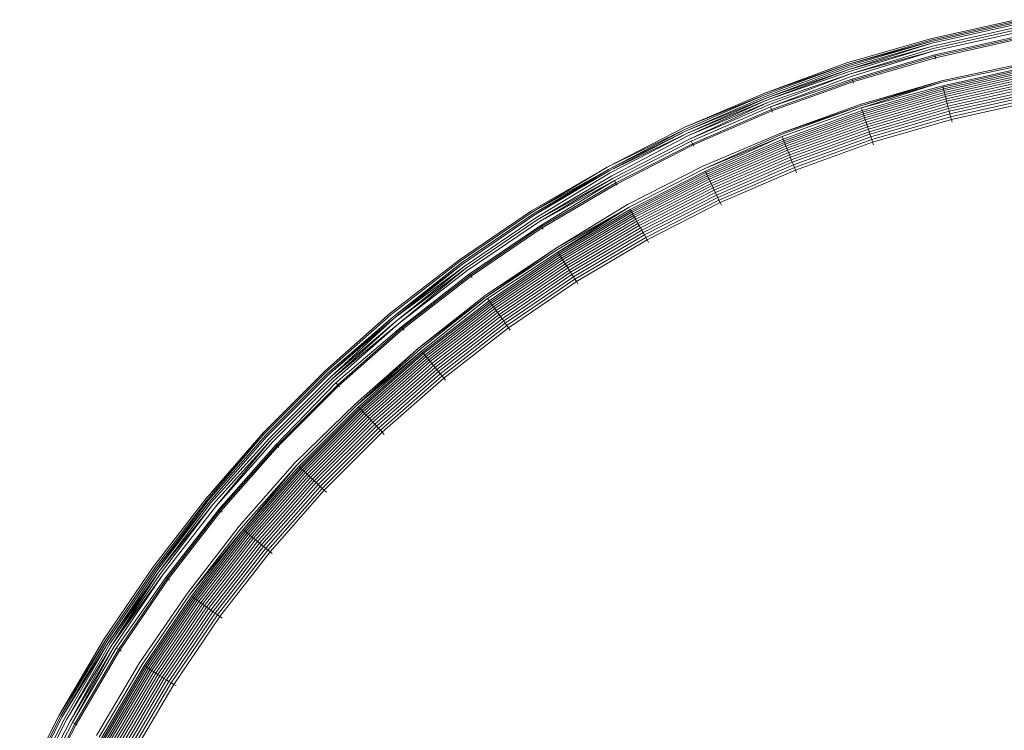
# Model space of a CAD drawing. Units: inches. Extents: x 64 to 1167, y 117 to 939.
# Tile 47 of 56: x 1129.2346 to 1130.0344, y 501.4737 to 502.0509. Entities that reach past the tile are written whole.
import ezdxf

# ---------------------------------------------------------------- set-up
doc = ezdxf.new("R2010")
doc.units = ezdxf.units.IN
doc.header["$MEASUREMENT"] = 0
doc.layers.add('A-FLOR-FIXT', color=8, linetype='Continuous', lineweight=18)

msp = doc.modelspace()

# ---------------------------------------------------------------- linework, layer by layer
at = {"layer": 'A-FLOR-FIXT'}
for p, q in [((1130.04375, 502.05092), (1129.97458, 502.03545)), ((1130.04398, 502.04972), (1129.97488, 502.03427)), ((1130.04419, 502.04859), (1129.97517, 502.03316)), ((1130.04446, 502.0472), (1129.97552, 502.0318)), ((1130.04493, 502.04472), (1129.97615, 502.02935)), ((1130.04529, 502.04284), (1129.97663, 502.02749)), ((1130.04568, 502.04081), (1129.97714, 502.02549)), ((1129.97458, 502.03545), (1129.90644, 502.01593)), ((1129.97488, 502.03427), (1129.9069, 502.01452)), ((1129.97517, 502.03316), (1129.9069, 502.01452)), ((1129.97517, 502.03316), (1129.90725, 502.01342)), ((1129.97552, 502.0318), (1129.90769, 502.01209)), ((1129.97552, 502.0318), (1129.90819, 502.01054)), ((1130.0463, 502.03755), (1129.97796, 502.02228)), ((1130.04651, 502.03644), (1129.97825, 502.02118)), ((1130.04673, 502.03531), (1129.97853, 502.02006)), ((1129.97615, 502.02935), (1129.90819, 502.01054)), ((1129.97615, 502.02935), (1129.90876, 502.00879)), ((1129.97663, 502.02749), (1129.90938, 502.00689)), ((1129.97714, 502.02549), (1129.90938, 502.00689)), ((1129.97714, 502.02549), (1129.91004, 502.00487)), ((1129.90644, 502.01593), (1129.83996, 501.99136)), ((1129.97796, 502.02228), (1129.91072, 502.00274)), ((1129.97825, 502.02118), (1129.91108, 502.00166)), ((1129.97853, 502.02006), (1129.91143, 502.00057)), ((1129.97825, 502.02118), (1129.97796, 502.02228)), ((1129.97853, 502.02006), (1129.97825, 502.02118)), ((1129.97882, 502.01895), (1129.97853, 502.02006)), ((1130.05047, 502.01568), (1129.98337, 502.00121)), ((1129.9069, 502.01452), (1129.83996, 501.99136)), ((1129.9069, 502.01452), (1129.84049, 501.99003)), ((1129.90725, 502.01342), (1129.84096, 501.98884)), ((1129.90769, 502.01209), (1129.84152, 501.98743)), ((1129.90819, 502.01054), (1129.84152, 501.98743)), ((1129.90819, 502.01054), (1129.84216, 501.98581)), ((1129.90876, 502.00879), (1129.84216, 501.98581)), ((1129.90938, 502.00689), (1129.84286, 501.98403)), ((1129.90938, 502.00689), (1129.84362, 501.9821)), ((1130.05075, 502.01422), (1129.98367, 502.00006)), ((1130.05113, 502.01221), (1129.98438, 501.99729)), ((1130.05136, 502.01101), (1129.98468, 501.99611)), ((1130.05161, 502.00969), (1129.98502, 501.99481)), ((1130.05189, 502.00825), (1129.98538, 501.99339)), ((1130.05218, 502.0067), (1129.98577, 501.99186)), ((1129.91004, 502.00487), (1129.84443, 501.98007)), ((1129.91072, 502.00274), (1129.84443, 501.98007)), ((1129.91108, 502.00166), (1129.84526, 501.97797)), ((1129.91143, 502.00057), (1129.84569, 501.9769)), ((1129.91108, 502.00166), (1129.91072, 502.00274)), ((1129.91143, 502.00057), (1129.91108, 502.00166)), ((1129.91179, 501.99947), (1129.91143, 502.00057)), ((1129.98337, 502.00121), (1129.91745, 501.98206)), ((1129.98337, 502.00121), (1129.91781, 501.98092)), ((1129.98367, 502.00006), (1129.91781, 501.98092)), ((1129.98367, 502.00006), (1129.91836, 501.97924)), ((1130.0525, 502.00505), (1129.98619, 501.99023)), ((1130.05283, 502.00329), (1129.98664, 501.9885)), ((1130.05319, 502.00145), (1129.9871, 501.98668)), ((1130.05355, 501.99952), (1129.98759, 501.98478)), ((1129.83996, 501.99136), (1129.77479, 501.96353)), ((1129.98438, 501.99729), (1129.91836, 501.97924)), ((1129.98468, 501.99611), (1129.91907, 501.97705)), ((1129.98502, 501.99481), (1129.91949, 501.97577)), ((1129.98538, 501.99339), (1129.91994, 501.97438)), ((1129.98577, 501.99186), (1129.92043, 501.97287)), ((1129.98438, 501.99729), (1129.98468, 501.99611)), ((1129.98468, 501.99611), (1129.98502, 501.99481)), ((1129.98502, 501.99481), (1129.98538, 501.99339)), ((1129.98538, 501.99339), (1129.98577, 501.99186)), ((1129.98577, 501.99186), (1129.98619, 501.99023)), ((1130.05393, 501.99752), (1129.9881, 501.98281)), ((1130.05433, 501.99546), (1129.98862, 501.98077)), ((1130.05473, 501.99333), (1129.98916, 501.97868)), ((1130.05515, 501.99116), (1129.98971, 501.97653)), ((1129.84049, 501.99003), (1129.77479, 501.96353)), ((1129.84049, 501.99003), (1129.77554, 501.96193)), ((1129.84096, 501.98884), (1129.77609, 501.96077)), ((1129.84152, 501.98743), (1129.77609, 501.96077)), ((1129.84152, 501.98743), (1129.77709, 501.95863)), ((1129.84216, 501.98581), (1129.77709, 501.95863)), ((1129.84216, 501.98581), (1129.77787, 501.95697)), ((1129.84286, 501.98403), (1129.77787, 501.95697)), ((1129.84286, 501.98403), (1129.77917, 501.95421)), ((1129.98619, 501.99023), (1129.92095, 501.97127)), ((1129.98664, 501.9885), (1129.9215, 501.96957)), ((1129.9871, 501.98668), (1129.92208, 501.96779)), ((1129.98759, 501.98478), (1129.92269, 501.96592)), ((1129.9881, 501.98281), (1129.92332, 501.96399)), ((1129.98619, 501.99023), (1129.98664, 501.9885)), ((1129.9871, 501.98668), (1129.98664, 501.9885)), ((1129.98759, 501.98478), (1129.9871, 501.98668)), ((1129.9881, 501.98281), (1129.98759, 501.98478)), ((1129.98862, 501.98077), (1129.9881, 501.98281)), ((1130.05557, 501.98895), (1129.99027, 501.97436)), ((1130.056, 501.98671), (1129.99084, 501.97215)), ((1130.05643, 501.98446), (1129.99141, 501.96992)), ((1129.84362, 501.9821), (1129.77917, 501.95421)), ((1129.84443, 501.98007), (1129.7801, 501.95224)), ((1129.84526, 501.97797), (1129.78107, 501.95019)), ((1129.84569, 501.9769), (1129.78156, 501.94915)), ((1129.84443, 501.98007), (1129.84526, 501.97797)), ((1129.84526, 501.97797), (1129.84569, 501.9769)), ((1129.84569, 501.9769), (1129.84611, 501.97583)), ((1129.91745, 501.98206), (1129.85285, 501.9588)), ((1129.91781, 501.98092), (1129.85285, 501.9588)), ((1129.91781, 501.98092), (1129.85329, 501.95769)), ((1129.91836, 501.97924), (1129.85394, 501.95605)), ((1129.91907, 501.97705), (1129.85479, 501.9539)), ((1129.91949, 501.97577), (1129.85529, 501.95265)), ((1129.91907, 501.97705), (1129.91836, 501.97924)), ((1129.91949, 501.97577), (1129.91907, 501.97705)), ((1129.91994, 501.97438), (1129.91949, 501.97577)), ((1129.98862, 501.98077), (1129.92397, 501.96198)), ((1129.98916, 501.97868), (1129.92464, 501.95993)), ((1129.98971, 501.97653), (1129.92532, 501.95783)), ((1129.98916, 501.97868), (1129.98862, 501.98077)), ((1129.98971, 501.97653), (1129.98916, 501.97868)), ((1129.99027, 501.97436), (1129.98971, 501.97653)), ((1129.91994, 501.97438), (1129.85582, 501.95129)), ((1129.92043, 501.97287), (1129.85641, 501.94982)), ((1129.92095, 501.97127), (1129.85703, 501.94826)), ((1129.9215, 501.96957), (1129.85768, 501.9466)), ((1129.92208, 501.96779), (1129.85837, 501.94485)), ((1129.92043, 501.97287), (1129.91994, 501.97438)), ((1129.92095, 501.97127), (1129.92043, 501.97287)), ((1129.9215, 501.96957), (1129.92095, 501.97127)), ((1129.92208, 501.96779), (1129.9215, 501.96957)), ((1129.92269, 501.96592), (1129.92208, 501.96779)), ((1129.99027, 501.97436), (1129.92601, 501.95569)), ((1129.99084, 501.97215), (1129.92672, 501.95352)), ((1129.99141, 501.96992), (1129.92743, 501.95134)), ((1129.99084, 501.97215), (1129.99027, 501.97436)), ((1129.99141, 501.96992), (1129.99084, 501.97215)), ((1129.99198, 501.96769), (1129.99141, 501.96992)), ((1129.77479, 501.96353), (1129.7118, 501.93106)), ((1129.77554, 501.96193), (1129.7118, 501.93106)), ((1129.77554, 501.96193), (1129.71278, 501.92927)), ((1129.77609, 501.96077), (1129.71278, 501.92927)), ((1129.77609, 501.96077), (1129.71346, 501.92804)), ((1129.77709, 501.95863), (1129.71346, 501.92804)), ((1129.77709, 501.95863), (1129.71425, 501.92661)), ((1129.85285, 501.9588), (1129.78959, 501.93208)), ((1129.92269, 501.96592), (1129.8591, 501.94303)), ((1129.92332, 501.96399), (1129.85985, 501.94113)), ((1129.92397, 501.96198), (1129.86062, 501.93918)), ((1129.92464, 501.95993), (1129.86142, 501.93717)), ((1129.92332, 501.96399), (1129.92269, 501.96592)), ((1129.92397, 501.96198), (1129.92332, 501.96399)), ((1129.92464, 501.95993), (1129.92397, 501.96198)), ((1129.92532, 501.95783), (1129.92464, 501.95993)), ((1129.77787, 501.95697), (1129.7156, 501.92414)), ((1129.77917, 501.95421), (1129.7166, 501.92233)), ((1129.7801, 501.95224), (1129.71765, 501.92042)), ((1129.78107, 501.95019), (1129.7801, 501.95224)), ((1129.85329, 501.95769), (1129.7907, 501.92972)), ((1129.85394, 501.95605), (1129.7907, 501.92972)), ((1129.85394, 501.95605), (1129.79157, 501.92787)), ((1129.85479, 501.9539), (1129.79209, 501.92677)), ((1129.85529, 501.95265), (1129.79266, 501.92555)), ((1129.85582, 501.95129), (1129.79328, 501.92423)), ((1129.85394, 501.95605), (1129.85479, 501.9539)), ((1129.85479, 501.9539), (1129.85529, 501.95265)), ((1129.85529, 501.95265), (1129.85582, 501.95129)), ((1129.85582, 501.95129), (1129.85641, 501.94982)), ((1129.92532, 501.95783), (1129.86223, 501.93511)), ((1129.92601, 501.95569), (1129.86306, 501.93302)), ((1129.92672, 501.95352), (1129.8639, 501.9309)), ((1129.92743, 501.95134), (1129.86474, 501.92877)), ((1129.92601, 501.95569), (1129.92532, 501.95783)), ((1129.92672, 501.95352), (1129.92601, 501.95569)), ((1129.92743, 501.95134), (1129.92672, 501.95352)), ((1129.92814, 501.94914), (1129.92743, 501.95134)), ((1129.78107, 501.95019), (1129.71874, 501.91843)), ((1129.78156, 501.94915), (1129.7193, 501.91742)), ((1129.78107, 501.95019), (1129.78156, 501.94915)), ((1129.78205, 501.9481), (1129.78156, 501.94915)), ((1129.85641, 501.94982), (1129.79396, 501.9228)), ((1129.85703, 501.94826), (1129.79467, 501.92127)), ((1129.85768, 501.9466), (1129.79543, 501.91966)), ((1129.85837, 501.94485), (1129.79623, 501.91796)), ((1129.8591, 501.94303), (1129.79707, 501.91619)), ((1129.85641, 501.94982), (1129.85703, 501.94826)), ((1129.85703, 501.94826), (1129.85768, 501.9466)), ((1129.85768, 501.9466), (1129.85837, 501.94485)), ((1129.85837, 501.94485), (1129.8591, 501.94303)), ((1129.8591, 501.94303), (1129.85985, 501.94113)), ((1129.85985, 501.94113), (1129.79793, 501.91434)), ((1129.86062, 501.93918), (1129.79883, 501.91244)), ((1129.86142, 501.93717), (1129.79975, 501.91048)), ((1129.86223, 501.93511), (1129.80069, 501.90848)), ((1129.85985, 501.94113), (1129.86062, 501.93918)), ((1129.86062, 501.93918), (1129.86142, 501.93717)), ((1129.86142, 501.93717), (1129.86223, 501.93511)), ((1129.86223, 501.93511), (1129.86306, 501.93302)), ((1129.7118, 501.93106), (1129.65039, 501.89565)), ((1129.7118, 501.93106), (1129.65103, 501.89464)), ((1129.71278, 501.92927), (1129.65103, 501.89464)), ((1129.71278, 501.92927), (1129.65191, 501.89327)), ((1129.71278, 501.92927), (1129.65266, 501.89208)), ((1129.71346, 501.92804), (1129.65266, 501.89208)), ((1129.78959, 501.93208), (1129.72838, 501.9009)), ((1129.7907, 501.92972), (1129.72964, 501.89861)), ((1129.79157, 501.92787), (1129.73062, 501.89682)), ((1129.79209, 501.92677), (1129.73121, 501.89575)), ((1129.79209, 501.92677), (1129.79157, 501.92787)), ((1129.79266, 501.92555), (1129.79209, 501.92677)), ((1129.86306, 501.93302), (1129.80165, 501.90645)), ((1129.8639, 501.9309), (1129.80262, 501.90439)), ((1129.86474, 501.92877), (1129.8036, 501.90231)), ((1129.86306, 501.93302), (1129.8639, 501.9309)), ((1129.8639, 501.9309), (1129.86474, 501.92877)), ((1129.86474, 501.92877), (1129.86559, 501.92662)), ((1129.71425, 501.92661), (1129.65401, 501.88995)), ((1129.7156, 501.92414), (1129.65504, 501.88833)), ((1129.7166, 501.92233), (1129.65504, 501.88833)), ((1129.7166, 501.92233), (1129.65615, 501.88658)), ((1129.71765, 501.92042), (1129.65615, 501.88658)), ((1129.71765, 501.92042), (1129.65792, 501.88379)), ((1129.71765, 501.92042), (1129.71874, 501.91843)), ((1129.79266, 501.92555), (1129.73186, 501.89457)), ((1129.79328, 501.92423), (1129.73256, 501.89329)), ((1129.79396, 501.9228), (1129.73332, 501.89191)), ((1129.79467, 501.92127), (1129.73414, 501.89043)), ((1129.79543, 501.91966), (1129.735, 501.88886)), ((1129.79328, 501.92423), (1129.79266, 501.92555)), ((1129.79396, 501.9228), (1129.79328, 501.92423)), ((1129.79467, 501.92127), (1129.79396, 501.9228)), ((1129.79543, 501.91966), (1129.79467, 501.92127)), ((1129.79623, 501.91796), (1129.79543, 501.91966)), ((1129.71874, 501.91843), (1129.65853, 501.88282)), ((1129.7193, 501.91742), (1129.65915, 501.88185)), ((1129.7193, 501.91742), (1129.71874, 501.91843)), ((1129.7193, 501.91742), (1129.71985, 501.91641)), ((1129.79623, 501.91796), (1129.7359, 501.88722)), ((1129.79707, 501.91619), (1129.73685, 501.8855)), ((1129.79793, 501.91434), (1129.73783, 501.88372)), ((1129.79883, 501.91244), (1129.73884, 501.88187)), ((1129.79707, 501.91619), (1129.79623, 501.91796)), ((1129.79793, 501.91434), (1129.79707, 501.91619)), ((1129.79883, 501.91244), (1129.79793, 501.91434)), ((1129.79975, 501.91048), (1129.79883, 501.91244)), ((1129.79975, 501.91048), (1129.73988, 501.87998)), ((1129.80069, 501.90848), (1129.74095, 501.87804)), ((1129.80165, 501.90645), (1129.74203, 501.87607)), ((1129.80262, 501.90439), (1129.74313, 501.87407)), ((1129.80069, 501.90848), (1129.79975, 501.91048)), ((1129.80165, 501.90645), (1129.80069, 501.90848)), ((1129.80262, 501.90439), (1129.80165, 501.90645)), ((1129.8036, 501.90231), (1129.80262, 501.90439)), ((1129.65039, 501.89565), (1129.59175, 501.8558)), ((1129.65103, 501.89464), (1129.59245, 501.85483)), ((1129.72838, 501.9009), (1129.66986, 501.86498)), ((1129.72964, 501.89861), (1129.66986, 501.86498)), ((1129.72964, 501.89861), (1129.67065, 501.86373)), ((1129.72964, 501.89861), (1129.67175, 501.862)), ((1129.73062, 501.89682), (1129.67175, 501.862)), ((1129.73121, 501.89575), (1129.6724, 501.86097)), ((1129.73062, 501.89682), (1129.73121, 501.89575)), ((1129.73121, 501.89575), (1129.73186, 501.89457)), ((1129.8036, 501.90231), (1129.74423, 501.87206)), ((1129.80458, 501.90022), (1129.8036, 501.90231)), ((1129.65191, 501.89327), (1129.59341, 501.85351)), ((1129.65266, 501.89208), (1129.59424, 501.85238)), ((1129.65401, 501.88995), (1129.59572, 501.85033)), ((1129.65504, 501.88833), (1129.59685, 501.84878)), ((1129.73186, 501.89457), (1129.67312, 501.85984)), ((1129.73256, 501.89329), (1129.67391, 501.8586)), ((1129.73332, 501.89191), (1129.67475, 501.85727)), ((1129.73414, 501.89043), (1129.67566, 501.85584)), ((1129.735, 501.88886), (1129.67661, 501.85434)), ((1129.7359, 501.88722), (1129.67762, 501.85275)), ((1129.73186, 501.89457), (1129.73256, 501.89329)), ((1129.73256, 501.89329), (1129.73332, 501.89191)), ((1129.73332, 501.89191), (1129.73414, 501.89043)), ((1129.73414, 501.89043), (1129.735, 501.88886)), ((1129.735, 501.88886), (1129.7359, 501.88722)), ((1129.7359, 501.88722), (1129.73685, 501.8855)), ((1129.65615, 501.88658), (1129.59807, 501.84711)), ((1129.65792, 501.88379), (1129.60001, 501.84443)), ((1129.65853, 501.88282), (1129.60068, 501.84351)), ((1129.65915, 501.88185), (1129.60136, 501.84258)), ((1129.65853, 501.88282), (1129.65792, 501.88379)), ((1129.65853, 501.88282), (1129.65915, 501.88185)), ((1129.65977, 501.88088), (1129.65915, 501.88185)), ((1129.73685, 501.8855), (1129.67867, 501.8511)), ((1129.73783, 501.88372), (1129.67976, 501.84938)), ((1129.73884, 501.88187), (1129.68089, 501.8476)), ((1129.73988, 501.87998), (1129.68205, 501.84578)), ((1129.73685, 501.8855), (1129.73783, 501.88372)), ((1129.73783, 501.88372), (1129.73884, 501.88187)), ((1129.73884, 501.88187), (1129.73988, 501.87998)), ((1129.73988, 501.87998), (1129.74095, 501.87804)), ((1129.74095, 501.87804), (1129.68323, 501.84391)), ((1129.74203, 501.87607), (1129.68444, 501.84201)), ((1129.74313, 501.87407), (1129.68566, 501.84009)), ((1129.74423, 501.87206), (1129.68689, 501.83815)), ((1129.74095, 501.87804), (1129.74203, 501.87607)), ((1129.74203, 501.87607), (1129.74313, 501.87407)), ((1129.74313, 501.87407), (1129.74423, 501.87206)), ((1129.74423, 501.87206), (1129.74535, 501.87004)), ((1129.66986, 501.86498), (1129.6128, 501.82683)), ((1129.66986, 501.86498), (1129.6135, 501.82587)), ((1129.67065, 501.86373), (1129.6135, 501.82587)), ((1129.59175, 501.8558), (1129.53566, 501.81243)), ((1129.59245, 501.85483), (1129.53649, 501.81142)), ((1129.67175, 501.862), (1129.61454, 501.82444)), ((1129.6724, 501.86097), (1129.61589, 501.82257)), ((1129.67312, 501.85984), (1129.61668, 501.82148)), ((1129.67391, 501.8586), (1129.61755, 501.8203)), ((1129.67475, 501.85727), (1129.61847, 501.81902)), ((1129.67566, 501.85584), (1129.61946, 501.81766)), ((1129.6724, 501.86097), (1129.67175, 501.862)), ((1129.67312, 501.85984), (1129.6724, 501.86097)), ((1129.67391, 501.8586), (1129.67312, 501.85984)), ((1129.67475, 501.85727), (1129.67391, 501.8586)), ((1129.67566, 501.85584), (1129.67475, 501.85727)), ((1129.67661, 501.85434), (1129.67566, 501.85584)), ((1129.59341, 501.85351), (1129.53796, 501.80965)), ((1129.59424, 501.85238), (1129.53796, 501.80965)), ((1129.59424, 501.85238), (1129.53893, 501.80847)), ((1129.59572, 501.85033), (1129.53893, 501.80847)), ((1129.59572, 501.85033), (1129.54063, 501.80641)), ((1129.59685, 501.84878), (1129.54063, 501.80641)), ((1129.59685, 501.84878), (1129.54258, 501.80406)), ((1129.59807, 501.84711), (1129.54258, 501.80406)), ((1129.67661, 501.85434), (1129.62051, 501.81621)), ((1129.67762, 501.85275), (1129.62162, 501.81469)), ((1129.67867, 501.8511), (1129.62277, 501.81311)), ((1129.67976, 501.84938), (1129.62397, 501.81146)), ((1129.68089, 501.8476), (1129.6252, 501.80976)), ((1129.67661, 501.85434), (1129.67762, 501.85275)), ((1129.67762, 501.85275), (1129.67867, 501.8511)), ((1129.67867, 501.8511), (1129.67976, 501.84938)), ((1129.67976, 501.84938), (1129.68089, 501.8476)), ((1129.68089, 501.8476), (1129.68205, 501.84578)), ((1129.60001, 501.84443), (1129.54469, 501.80151)), ((1129.60068, 501.84351), (1129.54541, 501.80064)), ((1129.60136, 501.84258), (1129.54614, 501.79975)), ((1129.60001, 501.84443), (1129.60068, 501.84351)), ((1129.60136, 501.84258), (1129.60068, 501.84351)), ((1129.60136, 501.84258), (1129.60204, 501.84164)), ((1129.68205, 501.84578), (1129.62647, 501.80801)), ((1129.68323, 501.84391), (1129.62777, 501.80622)), ((1129.68444, 501.84201), (1129.62909, 501.8044)), ((1129.68566, 501.84009), (1129.63043, 501.80256)), ((1129.68205, 501.84578), (1129.68323, 501.84391)), ((1129.68323, 501.84391), (1129.68444, 501.84201)), ((1129.68444, 501.84201), (1129.68566, 501.84009)), ((1129.68566, 501.84009), (1129.68689, 501.83815)), ((1129.68689, 501.83815), (1129.63178, 501.8007)), ((1129.68813, 501.8362), (1129.68689, 501.83815)), ((1129.6128, 501.82683), (1129.55888, 501.78435)), ((1129.6135, 501.82587), (1129.55888, 501.78435)), ((1129.6135, 501.82587), (1129.55983, 501.78321)), ((1129.61454, 501.82444), (1129.56113, 501.78163)), ((1129.61589, 501.82257), (1129.61454, 501.82444)), ((1129.61589, 501.82257), (1129.56191, 501.78069)), ((1129.61668, 501.82148), (1129.56277, 501.77966)), ((1129.61755, 501.8203), (1129.5637, 501.77853)), ((1129.61847, 501.81902), (1129.56471, 501.77731)), ((1129.61946, 501.81766), (1129.56578, 501.77601)), ((1129.62051, 501.81621), (1129.56692, 501.77464)), ((1129.62162, 501.81469), (1129.56811, 501.77319)), ((1129.61668, 501.82148), (1129.61589, 501.82257)), ((1129.61755, 501.8203), (1129.61668, 501.82148)), ((1129.61847, 501.81902), (1129.61755, 501.8203)), ((1129.61946, 501.81766), (1129.61847, 501.81902)), ((1129.62051, 501.81621), (1129.61946, 501.81766)), ((1129.62162, 501.81469), (1129.62051, 501.81621)), ((1129.62277, 501.81311), (1129.62162, 501.81469)), ((1129.53566, 501.81243), (1129.48254, 501.76545)), ((1129.53649, 501.81142), (1129.48336, 501.76458)), ((1129.53796, 501.80965), (1129.48448, 501.76339)), ((1129.53796, 501.80965), (1129.48544, 501.76237)), ((1129.53893, 501.80847), (1129.48544, 501.76237)), ((1129.53893, 501.80847), (1129.48717, 501.76053)), ((1129.62277, 501.81311), (1129.56936, 501.77168)), ((1129.62397, 501.81146), (1129.57066, 501.77011)), ((1129.6252, 501.80976), (1129.572, 501.76849)), ((1129.62647, 501.80801), (1129.57338, 501.76683)), ((1129.62397, 501.81146), (1129.62277, 501.81311)), ((1129.6252, 501.80976), (1129.62397, 501.81146)), ((1129.62647, 501.80801), (1129.6252, 501.80976)), ((1129.62777, 501.80622), (1129.62647, 501.80801)), ((1129.54063, 501.80641), (1129.48717, 501.76053)), ((1129.54063, 501.80641), (1129.48848, 501.75913)), ((1129.54258, 501.80406), (1129.48848, 501.75913)), ((1129.54258, 501.80406), (1129.4899, 501.75762)), ((1129.54469, 501.80151), (1129.49139, 501.75603)), ((1129.54541, 501.80064), (1129.49294, 501.75438)), ((1129.54614, 501.79975), (1129.49373, 501.75354)), ((1129.54469, 501.80151), (1129.54541, 501.80064)), ((1129.54541, 501.80064), (1129.54614, 501.79975)), ((1129.54614, 501.79975), (1129.54688, 501.79886)), ((1129.62777, 501.80622), (1129.57479, 501.76512)), ((1129.62909, 501.8044), (1129.57622, 501.76339)), ((1129.63043, 501.80256), (1129.57768, 501.76163)), ((1129.63178, 501.8007), (1129.57914, 501.75986)), ((1129.62909, 501.8044), (1129.62777, 501.80622)), ((1129.63043, 501.80256), (1129.62909, 501.8044)), ((1129.63178, 501.8007), (1129.63043, 501.80256)), ((1129.63178, 501.8007), (1129.63314, 501.79883)), ((1129.55888, 501.78435), (1129.50741, 501.73897)), ((1129.55888, 501.78435), (1129.50843, 501.73789)), ((1129.55983, 501.78321), (1129.50843, 501.73789)), ((1129.56113, 501.78163), (1129.50843, 501.73789)), ((1129.56113, 501.78163), (1129.50982, 501.7364)), ((1129.56191, 501.78069), (1129.51066, 501.73551)), ((1129.56277, 501.77966), (1129.51158, 501.73453)), ((1129.5637, 501.77853), (1129.51258, 501.73346)), ((1129.56471, 501.77731), (1129.51366, 501.73231)), ((1129.56578, 501.77601), (1129.51482, 501.73108)), ((1129.56113, 501.78163), (1129.56191, 501.78069)), ((1129.56191, 501.78069), (1129.56277, 501.77966)), ((1129.56277, 501.77966), (1129.5637, 501.77853)), ((1129.5637, 501.77853), (1129.56471, 501.77731)), ((1129.56471, 501.77731), (1129.56578, 501.77601)), ((1129.56578, 501.77601), (1129.56692, 501.77464)), ((1129.56692, 501.77464), (1129.51604, 501.72978)), ((1129.56811, 501.77319), (1129.51732, 501.72841)), ((1129.56936, 501.77168), (1129.51867, 501.72698)), ((1129.57066, 501.77011), (1129.52006, 501.7255)), ((1129.572, 501.76849), (1129.5215, 501.72397)), ((1129.57338, 501.76683), (1129.52298, 501.72239)), ((1129.56692, 501.77464), (1129.56811, 501.77319)), ((1129.56811, 501.77319), (1129.56936, 501.77168)), ((1129.56936, 501.77168), (1129.57066, 501.77011)), ((1129.57066, 501.77011), (1129.572, 501.76849)), ((1129.572, 501.76849), (1129.57338, 501.76683)), ((1129.57338, 501.76683), (1129.57479, 501.76512)), ((1129.48254, 501.76545), (1129.43241, 501.71532)), ((1129.48336, 501.76458), (1129.43328, 501.7145)), ((1129.48448, 501.76339), (1129.43446, 501.71338)), ((1129.48544, 501.76237), (1129.43549, 501.71242)), ((1129.48717, 501.76053), (1129.43733, 501.71069)), ((1129.48848, 501.75913), (1129.43873, 501.70938)), ((1129.57479, 501.76512), (1129.52449, 501.72078)), ((1129.57622, 501.76339), (1129.52603, 501.71914)), ((1129.57768, 501.76163), (1129.52759, 501.71748)), ((1129.57914, 501.75986), (1129.52917, 501.7158)), ((1129.57479, 501.76512), (1129.57622, 501.76339)), ((1129.57622, 501.76339), (1129.57768, 501.76163)), ((1129.57768, 501.76163), (1129.57914, 501.75986)), ((1129.57914, 501.75986), (1129.58061, 501.75808)), ((1129.4899, 501.75762), (1129.44024, 501.70796)), ((1129.49139, 501.75603), (1129.44265, 501.7057)), ((1129.49294, 501.75438), (1129.44348, 501.70492)), ((1129.49373, 501.75354), (1129.44432, 501.70413)), ((1129.49294, 501.75438), (1129.49139, 501.75603)), ((1129.49373, 501.75354), (1129.49294, 501.75438)), ((1129.49452, 501.7527), (1129.49373, 501.75354)), ((1129.50741, 501.73897), (1129.45823, 501.69107)), ((1129.50843, 501.73789), (1129.45997, 501.68943)), ((1129.50982, 501.7364), (1129.46146, 501.68804)), ((1129.51066, 501.73551), (1129.46235, 501.6872)), ((1129.51066, 501.73551), (1129.50982, 501.7364)), ((1129.51158, 501.73453), (1129.51066, 501.73551)), ((1129.51158, 501.73453), (1129.46333, 501.68628)), ((1129.51258, 501.73346), (1129.4644, 501.68528)), ((1129.51366, 501.73231), (1129.46555, 501.6842)), ((1129.51482, 501.73108), (1129.46677, 501.68304)), ((1129.51604, 501.72978), (1129.46808, 501.68182)), ((1129.51732, 501.72841), (1129.46944, 501.68054)), ((1129.51867, 501.72698), (1129.47087, 501.67919)), ((1129.51258, 501.73346), (1129.51158, 501.73453)), ((1129.51366, 501.73231), (1129.51258, 501.73346)), ((1129.51482, 501.73108), (1129.51366, 501.73231)), ((1129.51604, 501.72978), (1129.51482, 501.73108)), ((1129.51732, 501.72841), (1129.51604, 501.72978)), ((1129.51867, 501.72698), (1129.51732, 501.72841)), ((1129.52006, 501.7255), (1129.51867, 501.72698)), ((1129.52006, 501.7255), (1129.47236, 501.6778)), ((1129.5215, 501.72397), (1129.47389, 501.67636)), ((1129.52298, 501.72239), (1129.47547, 501.67488)), ((1129.52449, 501.72078), (1129.47708, 501.67337)), ((1129.52603, 501.71914), (1129.47872, 501.67183)), ((1129.52006, 501.7255), (1129.5215, 501.72397)), ((1129.5215, 501.72397), (1129.52298, 501.72239)), ((1129.52298, 501.72239), (1129.52449, 501.72078)), ((1129.52449, 501.72078), (1129.52603, 501.71914)), ((1129.52603, 501.71914), (1129.52759, 501.71748)), ((1129.43241, 501.71532), (1129.38586, 501.66184)), ((1129.43328, 501.7145), (1129.38586, 501.66184)), ((1129.43328, 501.7145), (1129.3868, 501.66107)), ((1129.43446, 501.71338), (1129.38769, 501.66033)), ((1129.43549, 501.71242), (1129.38878, 501.65944)), ((1129.43733, 501.71069), (1129.39003, 501.6584)), ((1129.52759, 501.71748), (1129.48038, 501.67027)), ((1129.52917, 501.7158), (1129.48206, 501.66869)), ((1129.52759, 501.71748), (1129.52917, 501.7158)), ((1129.52917, 501.7158), (1129.53075, 501.71412)), ((1129.43873, 501.70938), (1129.39144, 501.65723)), ((1129.43873, 501.70938), (1129.39379, 501.65528)), ((1129.44024, 501.70796), (1129.39379, 501.65528)), ((1129.44265, 501.7057), (1129.39635, 501.65317)), ((1129.44348, 501.70492), (1129.39722, 501.65245)), ((1129.44432, 501.70413), (1129.39811, 501.65171)), ((1129.44348, 501.70492), (1129.44265, 501.7057)), ((1129.44432, 501.70413), (1129.44348, 501.70492)), ((1129.44516, 501.70334), (1129.44432, 501.70413)), ((1129.45823, 501.69107), (1129.41281, 501.63955)), ((1129.45997, 501.68943), (1129.41465, 501.63803)), ((1129.45997, 501.68943), (1129.41622, 501.63673)), ((1129.46146, 501.68804), (1129.41622, 501.63673)), ((1129.46235, 501.6872), (1129.41716, 501.63595)), ((1129.46235, 501.6872), (1129.46146, 501.68804)), ((1129.46333, 501.68628), (1129.46235, 501.6872)), ((1129.46333, 501.68628), (1129.4182, 501.63509)), ((1129.4644, 501.68528), (1129.41933, 501.63416)), ((1129.46555, 501.6842), (1129.42055, 501.63315)), ((1129.46677, 501.68304), (1129.42184, 501.63208)), ((1129.46808, 501.68182), (1129.42322, 501.63094)), ((1129.46944, 501.68054), (1129.42467, 501.62974)), ((1129.47087, 501.67919), (1129.42618, 501.62849)), ((1129.4644, 501.68528), (1129.46333, 501.68628)), ((1129.46555, 501.6842), (1129.4644, 501.68528)), ((1129.46677, 501.68304), (1129.46555, 501.6842)), ((1129.46808, 501.68182), (1129.46677, 501.68304)), ((1129.46944, 501.68054), (1129.46808, 501.68182)), ((1129.47087, 501.67919), (1129.46944, 501.68054)), ((1129.47236, 501.6778), (1129.47087, 501.67919)), ((1129.47236, 501.6778), (1129.42775, 501.6272)), ((1129.47389, 501.67636), (1129.42937, 501.62585)), ((1129.47547, 501.67488), (1129.43103, 501.62448)), ((1129.47708, 501.67337), (1129.43274, 501.62307)), ((1129.47872, 501.67183), (1129.43447, 501.62163)), ((1129.47389, 501.67636), (1129.47236, 501.6778)), ((1129.47547, 501.67488), (1129.47389, 501.67636)), ((1129.47708, 501.67337), (1129.47547, 501.67488)), ((1129.47872, 501.67183), (1129.47708, 501.67337)), ((1129.48038, 501.67027), (1129.47872, 501.67183)), ((1129.48038, 501.67027), (1129.43622, 501.62018)), ((1129.48206, 501.66869), (1129.438, 501.61872)), ((1129.48206, 501.66869), (1129.48038, 501.67027)), ((1129.48374, 501.66711), (1129.48206, 501.66869)), ((1129.38586, 501.66184), (1129.34243, 501.60584)), ((1129.3868, 501.66107), (1129.34385, 501.60481)), ((1129.38769, 501.66033), (1129.34489, 501.60405)), ((1129.38878, 501.65944), (1129.34489, 501.60405)), ((1129.38878, 501.65944), (1129.34612, 501.60316)), ((1129.39003, 501.6584), (1129.34752, 501.60214)), ((1129.39144, 501.65723), (1129.34752, 501.60214)), ((1129.39144, 501.65723), (1129.34908, 501.60101)), ((1129.39379, 501.65528), (1129.35075, 501.59979)), ((1129.39635, 501.65317), (1129.35343, 501.59785)), ((1129.39722, 501.65245), (1129.35435, 501.59718)), ((1129.39811, 501.65171), (1129.35528, 501.5965)), ((1129.39635, 501.65317), (1129.39722, 501.65245)), ((1129.39722, 501.65245), (1129.39811, 501.65171)), ((1129.39811, 501.65171), (1129.399, 501.65098)), ((1129.41281, 501.63955), (1129.37103, 501.58506)), ((1129.41465, 501.63803), (1129.37265, 501.58388)), ((1129.41622, 501.63673), (1129.37265, 501.58388)), ((1129.41622, 501.63673), (1129.3743, 501.58268)), ((1129.41716, 501.63595), (1129.37529, 501.58197)), ((1129.4182, 501.63509), (1129.37638, 501.58117)), ((1129.41933, 501.63416), (1129.37756, 501.58031)), ((1129.42055, 501.63315), (1129.37884, 501.57939)), ((1129.42184, 501.63208), (1129.3802, 501.57839)), ((1129.42322, 501.63094), (1129.38165, 501.57735)), ((1129.41716, 501.63595), (1129.41622, 501.63673)), ((1129.4182, 501.63509), (1129.41716, 501.63595)), ((1129.41933, 501.63416), (1129.4182, 501.63509)), ((1129.41933, 501.63416), (1129.42055, 501.63315)), ((1129.42184, 501.63208), (1129.42055, 501.63315)), ((1129.42184, 501.63208), (1129.42322, 501.63094)), ((1129.42322, 501.63094), (1129.42467, 501.62974)), ((1129.42467, 501.62974), (1129.38317, 501.57624)), ((1129.42618, 501.62849), (1129.38475, 501.57509)), ((1129.42775, 501.6272), (1129.3864, 501.57389)), ((1129.42937, 501.62585), (1129.3881, 501.57266)), ((1129.43103, 501.62448), (1129.38985, 501.57139)), ((1129.43274, 501.62307), (1129.39164, 501.57009)), ((1129.42467, 501.62974), (1129.42618, 501.62849)), ((1129.42618, 501.62849), (1129.42775, 501.6272)), ((1129.42937, 501.62585), (1129.42775, 501.6272)), ((1129.42937, 501.62585), (1129.43103, 501.62448)), ((1129.43103, 501.62448), (1129.43274, 501.62307)), ((1129.43274, 501.62307), (1129.43447, 501.62163)), ((1129.43447, 501.62163), (1129.39346, 501.56876)), ((1129.43622, 501.62018), (1129.3953, 501.56742)), ((1129.438, 501.61872), (1129.39716, 501.56607)), ((1129.43447, 501.62163), (1129.43622, 501.62018)), ((1129.43622, 501.62018), (1129.438, 501.61872)), ((1129.438, 501.61872), (1129.43977, 501.61725)), ((1129.34243, 501.60584), (1129.30259, 501.54722)), ((1129.34385, 501.60481), (1129.30408, 501.54628)), ((1129.34489, 501.60405), (1129.30516, 501.54559)), ((1129.34612, 501.60316), (1129.30644, 501.54478)), ((1129.34752, 501.60214), (1129.30644, 501.54478)), ((1129.34752, 501.60214), (1129.30791, 501.54385)), ((1129.34752, 501.60214), (1129.30953, 501.54282)), ((1129.34908, 501.60101), (1129.30953, 501.54282)), ((1129.35075, 501.59979), (1129.30953, 501.54282)), ((1129.35075, 501.59979), (1129.31128, 501.54171)), ((1129.35343, 501.59785), (1129.31312, 501.54054)), ((1129.35435, 501.59718), (1129.31503, 501.53932)), ((1129.35528, 501.5965), (1129.316, 501.53871)), ((1129.35435, 501.59718), (1129.35343, 501.59785)), ((1129.35528, 501.5965), (1129.35435, 501.59718)), ((1129.35621, 501.59582), (1129.35528, 501.5965)), ((1129.37103, 501.58506), (1129.33193, 501.5286)), ((1129.37265, 501.58388), (1129.33413, 501.5272)), ((1129.3743, 501.58268), (1129.33586, 501.52611)), ((1129.37529, 501.58197), (1129.33689, 501.52546)), ((1129.37638, 501.58117), (1129.33802, 501.52474)), ((1129.37756, 501.58031), (1129.33926, 501.52395)), ((1129.37884, 501.57939), (1129.34059, 501.52311)), ((1129.3802, 501.57839), (1129.34201, 501.5222)), ((1129.38165, 501.57735), (1129.34352, 501.52125)), ((1129.38317, 501.57624), (1129.34511, 501.52024)), ((1129.38475, 501.57509), (1129.34676, 501.51919)), ((1129.37529, 501.58197), (1129.3743, 501.58268)), ((1129.37638, 501.58117), (1129.37529, 501.58197)), ((1129.37756, 501.58031), (1129.37638, 501.58117)), ((1129.37884, 501.57939), (1129.37756, 501.58031)), ((1129.3802, 501.57839), (1129.37884, 501.57939)), ((1129.38165, 501.57735), (1129.3802, 501.57839)), ((1129.38317, 501.57624), (1129.38165, 501.57735)), ((1129.38475, 501.57509), (1129.38317, 501.57624)), ((1129.3864, 501.57389), (1129.38475, 501.57509)), ((1129.3864, 501.57389), (1129.34848, 501.5181)), ((1129.3881, 501.57266), (1129.35026, 501.51697)), ((1129.38985, 501.57139), (1129.35208, 501.51581)), ((1129.39164, 501.57009), (1129.35395, 501.51463)), ((1129.39346, 501.56876), (1129.35585, 501.51342)), ((1129.3953, 501.56742), (1129.35777, 501.5122)), ((1129.3881, 501.57266), (1129.3864, 501.57389)), ((1129.38985, 501.57139), (1129.3881, 501.57266)), ((1129.39164, 501.57009), (1129.38985, 501.57139)), ((1129.39346, 501.56876), (1129.39164, 501.57009)), ((1129.3953, 501.56742), (1129.39346, 501.56876)), ((1129.39716, 501.56607), (1129.3953, 501.56742)), ((1129.39716, 501.56607), (1129.35971, 501.51097)), ((1129.39903, 501.56472), (1129.39716, 501.56607)), ((1129.30259, 501.54722), (1129.2668, 501.48606)), ((1129.30408, 501.54628), (1129.2668, 501.48606)), ((1129.30408, 501.54628), (1129.26805, 501.48537)), ((1129.30516, 501.54559), (1129.26918, 501.48475)), ((1129.30644, 501.54478), (1129.26918, 501.48475)), ((1129.30644, 501.54478), (1129.27125, 501.48361)), ((1129.30791, 501.54385), (1129.27285, 501.48273)), ((1129.30953, 501.54282), (1129.27285, 501.48273)), ((1129.30953, 501.54282), (1129.27553, 501.48126)), ((1129.31128, 501.54171), (1129.27553, 501.48126)), ((1129.31128, 501.54171), (1129.27744, 501.48021)), ((1129.31312, 501.54054), (1129.27744, 501.48021)), ((1129.31503, 501.53932), (1129.27943, 501.47912)), ((1129.316, 501.53871), (1129.28043, 501.47856)), ((1129.31312, 501.54054), (1129.31503, 501.53932)), ((1129.31503, 501.53932), (1129.316, 501.53871)), ((1129.316, 501.53871), (1129.31698, 501.53809)), ((1129.33193, 501.5286), (1129.29696, 501.46948)), ((1129.33413, 501.5272), (1129.29925, 501.46822)), ((1129.33586, 501.52611), (1129.30104, 501.46724)), ((1129.33689, 501.52546), (1129.30211, 501.46665)), ((1129.33802, 501.52474), (1129.30328, 501.466)), ((1129.33926, 501.52395), (1129.30457, 501.46529)), ((1129.34059, 501.52311), (1129.30595, 501.46453)), ((1129.34201, 501.5222), (1129.30743, 501.46372)), ((1129.34352, 501.52125), (1129.30899, 501.46286)), ((1129.34511, 501.52024), (1129.31064, 501.46196)), ((1129.34676, 501.51919), (1129.31236, 501.46101)), ((1129.33689, 501.52546), (1129.33586, 501.52611)), ((1129.33802, 501.52474), (1129.33689, 501.52546)), ((1129.33926, 501.52395), (1129.33802, 501.52474)), ((1129.34059, 501.52311), (1129.33926, 501.52395)), ((1129.34201, 501.5222), (1129.34059, 501.52311)), ((1129.34352, 501.52125), (1129.34201, 501.5222)), ((1129.34511, 501.52024), (1129.34352, 501.52125)), ((1129.34676, 501.51919), (1129.34511, 501.52024)), ((1129.34848, 501.5181), (1129.34676, 501.51919)), ((1129.34848, 501.5181), (1129.31414, 501.46003)), ((1129.35026, 501.51697), (1129.31599, 501.45902)), ((1129.35208, 501.51581), (1129.31788, 501.45798)), ((1129.35395, 501.51463), (1129.31982, 501.45691)), ((1129.35585, 501.51342), (1129.32179, 501.45583)), ((1129.35777, 501.5122), (1129.32378, 501.45473)), ((1129.35971, 501.51097), (1129.3258, 501.45362)), ((1129.35026, 501.51697), (1129.34848, 501.5181)), ((1129.35208, 501.51581), (1129.35026, 501.51697)), ((1129.35395, 501.51463), (1129.35208, 501.51581)), ((1129.35585, 501.51342), (1129.35395, 501.51463)), ((1129.35777, 501.5122), (1129.35585, 501.51342)), ((1129.35971, 501.51097), (1129.35777, 501.5122)), ((1129.36166, 501.50973), (1129.35971, 501.51097)), ((1129.2668, 501.48606), (1129.23464, 501.42293)), ((1129.26805, 501.48537), (1129.23593, 501.42232)), ((1129.26918, 501.48475), (1129.23709, 501.42177)), ((1129.27125, 501.48361), (1129.23923, 501.42076)), ((1129.27285, 501.48273), (1129.24089, 501.41999)), ((1129.27553, 501.48126), (1129.24365, 501.41869)), ((1129.27744, 501.48021), (1129.24562, 501.41776)), ((1129.27943, 501.47912), (1129.24767, 501.41679)), ((1129.27943, 501.47912), (1129.27744, 501.48021)), ((1129.28043, 501.47856), (1129.27943, 501.47912)), ((1129.28043, 501.47856), (1129.24871, 501.4163)), ((1129.28145, 501.47801), (1129.28043, 501.47856))]:
    msp.add_line(p, q, dxfattribs=at)

doc.saveas('drawing.dxf')
